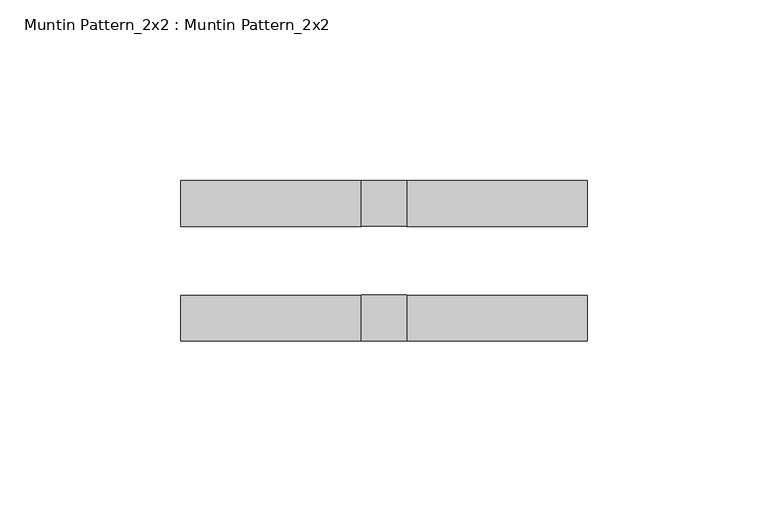
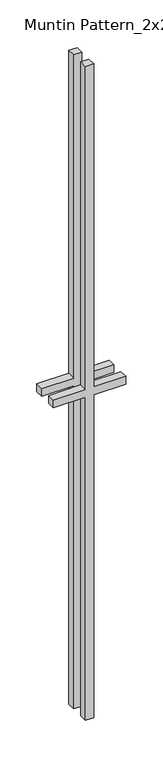
"""IFC4 building model written with IfcOpenShell, lengths in millimetres: proxy geometry, Muntin Pattern_2x2 : Muntin Pattern_2x2."""

from ifc_helpers import new_model, si_unit, frame, origin, place, context, project, spatial, polyline, outline, extrude, source, transform, mapped, element, save


def muntin_pattern_2x2_muntin_pattern_2x2_750a293b(model_context):
    return source(origin(), model_context, "Body", "SweptSolid", [
        extrude(outline(polyline([(546.1, -6.35), (546.1, -56.3378825), (533.4, -56.3378825), (533.4, -6.35), (0.0, -6.35), (0.0, 6.35), (533.4, 6.35), (533.4, 56.3378825), (546.1, 56.3378825), (546.1, 6.35), (1079.5, 6.35), (1079.5, -6.35), (546.1, -6.35)])), frame((0.0, 9.525, 0.0), z_axis=(0.0, 1.0, 0.0), x_axis=(0.0, 0.0, 1.0)), (0.0, 0.0, 1.0), 12.7),
        extrude(outline(polyline([(546.1, -6.35), (546.1, -56.3378825), (533.4, -56.3378825), (533.4, -6.35), (0.0, -6.35), (0.0, 6.35), (533.4, 6.35), (533.4, 56.3378825), (546.1, 56.3378825), (546.1, 6.35), (1079.5, 6.35), (1079.5, -6.35), (546.1, -6.35)])), frame((0.0, -22.225, 0.0), z_axis=(0.0, 1.0, 0.0), x_axis=(0.0, 0.0, 1.0)), (0.0, 0.0, 1.0), 12.7),
    ])


if __name__ == "__main__":
    model = new_model("IFC4")
    model_context = context("Model", 3, world=origin())
    ifc_project = project(units=[si_unit("LENGTHUNIT", "METRE", prefix="MILLI")], contexts=[model_context])
    site = spatial("IfcSite", under=ifc_project)
    building = spatial("IfcBuilding", under=site)
    placement = place(None, origin())
    muntin_pattern_2x2_muntin_pattern_2x2_shape = muntin_pattern_2x2_muntin_pattern_2x2_750a293b(model_context)
    element("IfcBuildingElementProxy", 1, Name="Muntin Pattern_2x2 : Muntin Pattern_2x2", ObjectType="Muntin Pattern_2x2 : Muntin Pattern_2x2", at=placement, inside=building, context=model_context, shape_type="MappedRepresentation", body=[
        mapped(muntin_pattern_2x2_muntin_pattern_2x2_shape, transform((0.0, 0.0, 0.0), x_axis=(1.0, 0.0, 0.0), y_axis=(0.0, 1.0, 0.0), z_axis=(0.0, 0.0, 1.0))),
    ])
    save(model, "model.ifc")

# Revit data of these elements
# Type "Muntin Pattern_2x2 : Muntin Pattern_2x2"
#   Width [instance default] = 4' - 0"
#   Thickness = 0' - 0 1/2"
#   Height [instance default] = 4' - 0"
#   Distance = 0' - 0 3/4"
#   Interior Material [instance default] = none
#   Exterior Material [instance default] = none
#   Default Elevation = 0
# Element 1 (IfcBuildingElementProxy, "Muntin Pattern_2x2 : Muntin Pattern_2x2")
#   Width = 0' - 4.43605"
#   Height = 3' - 6 1/2"
#   Interior Material = Wood - Stained
#   Exterior Material = Clad - White
#   Materials on its faces: "Clad - White", "Wood - Stained"
# Materials
#   "Clad - White": class "Wood", colour RGB 242 242 238, transparency 0, Cost = 0
#   "Wood - Stained": class "Wood", colour RGB 224 178 126, transparency 0, Cost = 0
